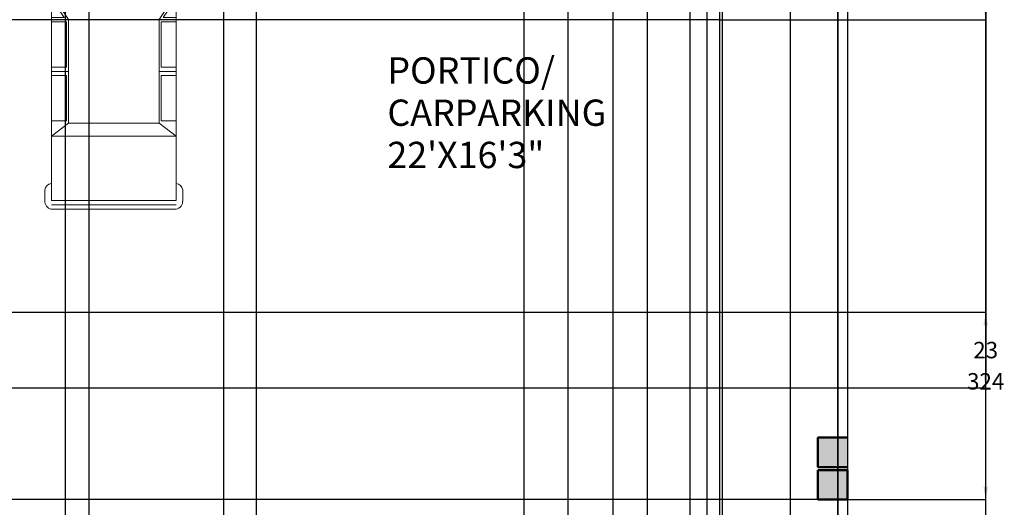
# Model space of a CAD drawing. Units: inches. Extents: x 460 to 1030, y -658 to 271.
# Tile 5 of 10: x 728 to 1028, y -488 to -340. Entities that reach past the tile are written whole.
import ezdxf

# ---------------------------------------------------------------- set-up
doc = ezdxf.new("R2010")
doc.units = ezdxf.units.IN
doc.header["$MEASUREMENT"] = 0
doc.linetypes.add('ACAD_ISO02W100', pattern=[15, 12, -3])
for name, color, linetype, lineweight in [('A-ANNO-DIMS', 2, 'Continuous', 18), ('A-AREA-IDEN', 7, 'Continuous', 25), ('A-COLS', 7, 'Continuous', 50), ('A-ROOF-OVHD', 8, 'ACAD_ISO02W100', 18), ('C-PROP', 7, 'Continuous', 25), ('C-SITE-VEHI', 8, 'Continuous', 13)]:
    doc.layers.add(name, color=color, linetype=linetype, lineweight=lineweight)
doc.layers.add('A-COLS-PATT', color=7, linetype='Continuous', lineweight=13, true_color=0xffffff)
doc.styles.get("Standard").update_dxf_attribs({"font": 'arial.ttf'})
doc.dimstyles.get("Standard").update_dxf_attribs({"dimtxt": 5, "dimasz": 4, "dimexe": 0.18, "dimexo": 0.0625, "dimgap": 0.09, "dimtad": 0, "dimtih": 1, "dimtoh": 1, "dimdec": 1, "dimzin": 0, "dimdsep": 46, "dimlunit": 4, "dimtxsty": 'Standard', "dimcen": 0.09, "dimadec": 0, "dimazin": 0, "dimtfac": 1, "dimtdec": 1, "dimtofl": 0, "dimtmove": 0, "dimatfit": 3, "dimfxl": 1, "dimtolj": 1, "dimtzin": 0, "dimarcsym": 0})

# ---------------------------------------------------------------- blocks, each defined once
blk = doc.blocks.new('*U14')
for p, q in [((3, -10), (3, 974)), ((70, -10), (70, 973)), ((138, 1075), (308, 1075)), ((138, 973), (410, 973)), ((138, -10), (138, 971)), ((410, 973), (4581, 973)), ((1563, -10), (1563, 973)), ((1563, 973), (1969, 702)), ((1630, 973), (1936, 769)), ((1936, 769), (1936, 973)), ((2003, 973), (2003, 736)), ((2716, 736), (2716, 973)), ((2783, 702), (2783, 973)), ((2851, 973), (2851, 736)), ((3563, 736), (3563, 973)), ((3597, 702), (3801, 973)), ((3801, -10), (3801, 973)), ((4818, 973), (4547, 973)), ((4818, 1075), (4649, 1075)), ((4818, -10), (4818, 971)), ((4886, -10), (4886, 973)), ((4954, -10), (4954, 974)), ((1969, 702), (3597, 702)), ((1969, -10), (1969, 702)), ((2003, 736), (2716, 736)), ((2851, 736), (3563, 736)), ((3597, -10), (3597, 702)), ((138, 193), (1563, 396)), ((3, -11), (3, -995)), ((70, -10), (70, -994)), ((138, -11), (138, -992)), ((1563, -10), (1563, -994)), ((1969, -10), (1969, -723)), ((3597, -10), (3597, -723)), ((3801, -10), (3801, -994)), ((4818, -11), (4818, -992)), ((4886, -10), (4886, -994)), ((4954, -11), (4954, -995)), ((138, -214), (1563, -417)), ((1563, -994), (1969, -723)), ((1969, -723), (3597, -723)), ((2003, -994), (2003, -757)), ((2003, -757), (2716, -757)), ((2716, -757), (2716, -994)), ((2783, -723), (2783, -994)), ((2851, -757), (3563, -757)), ((2851, -994), (2851, -757)), ((3563, -757), (3563, -994)), ((3597, -723), (3801, -994)), ((1630, -994), (1936, -790)), ((1936, -790), (1936, -994)), ((138, -994), (410, -994)), ((410, -994), (4581, -994)), ((4818, -994), (4547, -994)), ((138, -1096), (308, -1096)), ((4818, -1096), (4649, -1096))]:
    blk.add_line(p, q)
for centre, radius, start, end in [((128, 946), 129, 85.6455, 168.0943), ((291, 956), 120, 8.1301, 81.87), ((4665, 956), 120, 98.13, 171.8699), ((4828, 946), 129, 11.9057, 94.3545), ((128, -967), 129, 191.9057, 274.3545), ((291, -977), 120, 278.13, 351.8699), ((4665, -977), 120, 188.1301, 261.87), ((4828, -967), 129, 265.6455, 348.0943)]:
    blk.add_arc(centre, radius, start, end)
blk = doc.blocks.new('*D42')
at = {"layer": 'A-ANNO-DIMS', "color": 0, "lineweight": -2, "transparency": 16777216}
for p, q in [((940.86, -287.73), (1022.03, -287.73)), ((1021.85, -291.73), (1021.85, -447.08)), ((1021.85, -607.73), (1021.85, -452.37)), ((979.86, -611.73), (1022.03, -611.73))]:
    blk.add_line(p, q, dxfattribs=at)
at = {"layer": 'A-ANNO-DIMS', "color": 0, "transparency": 16777216}
for points in [[(1021.18, -291.73), (1022.51, -291.73), (1021.85, -287.73)], [(1021.18, -607.73), (1022.51, -607.73), (1021.85, -611.73)]]:
    blk.add_solid(points, dxfattribs=at)
at = {"layer": 'Defpoints', "color": 0, "transparency": 16777216}
for p in [(940.8, -287.73), (1021.85, -287.73), (979.8, -611.73)]:
    blk.add_point(p, dxfattribs=at)
at = {"layer": 'A-ANNO-DIMS', "color": 0, "transparency": 16777216, "insert": (1021.85, -449.73), "char_height": 5, "attachment_point": 5}
blk.add_mtext('\\A1;324', dxfattribs=at)
blk = doc.blocks.new('*D44')
at = {"layer": 'A-ANNO-DIMS', "color": 0, "lineweight": -2, "transparency": 16777216}
for p, q in [((940.86, 90.27), (1022.03, 90.27)), ((1021.85, 86.27), (1021.85, -195.08)), ((1021.85, -481.73), (1021.85, -200.37)), ((979.86, -485.73), (1022.03, -485.73))]:
    blk.add_line(p, q, dxfattribs=at)
at = {"layer": 'A-ANNO-DIMS', "color": 0, "transparency": 16777216}
for points in [[(1021.18, 86.27), (1022.51, 86.27), (1021.85, 90.27)], [(1021.18, -481.73), (1022.51, -481.73), (1021.85, -485.73)]]:
    blk.add_solid(points, dxfattribs=at)
at = {"layer": 'Defpoints', "color": 0, "transparency": 16777216}
for p in [(940.8, 90.27), (979.8, -485.73), (1021.85, -485.73)]:
    blk.add_point(p, dxfattribs=at)
at = {"layer": 'A-ANNO-DIMS', "color": 0, "transparency": 16777216, "insert": (1021.85, -197.73), "char_height": 5, "attachment_point": 5}
blk.add_mtext('\\A1;576', dxfattribs=at)
blk = doc.blocks.new('*D45')
at = {"layer": 'A-ANNO-DIMS', "color": 0, "lineweight": -2, "transparency": 16777216}
for p, q in [((976.8, 126.21), (976.8, -654.61)), ((940.8, 90.21), (940.8, -654.61)), ((944.8, -654.43), (955.13, -654.43)), ((972.8, -654.43), (962.46, -654.43))]:
    blk.add_line(p, q, dxfattribs=at)
at = {"layer": 'A-ANNO-DIMS', "color": 0, "transparency": 16777216}
for points in [[(944.8, -653.77), (944.8, -655.1), (940.8, -654.43)], [(972.8, -653.77), (972.8, -655.1), (976.8, -654.43)]]:
    blk.add_solid(points, dxfattribs=at)
at = {"layer": 'Defpoints', "color": 0, "transparency": 16777216}
for p in [(976.8, 126.27), (940.8, 90.27), (976.8, -654.43)]:
    blk.add_point(p, dxfattribs=at)
at = {"layer": 'A-ANNO-DIMS', "color": 0, "transparency": 16777216, "insert": (958.8, -654.43), "char_height": 5, "attachment_point": 5}
blk.add_mtext('\\A1;36', dxfattribs=at)
blk = doc.blocks.new('*D46')
at = {"layer": 'A-ANNO-DIMS', "color": 0, "lineweight": -2, "transparency": 16777216}
for p, q in [((936.98, 127.21), (936.98, -654.61)), ((962.32, 127.21), (962.32, -654.61)), ((932.98, -654.43), (928.98, -654.43)), ((966.32, -654.43), (970.32, -654.43))]:
    blk.add_line(p, q, dxfattribs=at)
at = {"layer": 'A-ANNO-DIMS', "color": 0, "transparency": 16777216}
for points in [[(932.98, -653.77), (932.98, -655.1), (936.98, -654.43)], [(966.32, -653.77), (966.32, -655.1), (962.32, -654.43)]]:
    blk.add_solid(points, dxfattribs=at)
at = {"layer": 'Defpoints', "color": 0, "transparency": 16777216}
for p in [(936.98, 127.27), (962.32, 127.27), (962.32, -654.43)]:
    blk.add_point(p, dxfattribs=at)
at = {"layer": 'A-ANNO-DIMS', "color": 0, "transparency": 16777216, "insert": (949.65, -654.43), "char_height": 5, "attachment_point": 5}
blk.add_mtext('\\A1;25.346', dxfattribs=at)
blk = doc.blocks.new('*D47')
at = {"layer": 'A-ANNO-DIMS', "color": 0, "lineweight": -2, "transparency": 16777216}
for p, q in [((962.32, 129.21), (962.32, -654.61)), ((979.8, 129.21), (979.8, -654.61)), ((966.32, -654.43), (975.8, -654.43)), ((979.8, -654.43), (983.8, -654.43))]:
    blk.add_line(p, q, dxfattribs=at)
at = {"layer": 'A-ANNO-DIMS', "color": 0, "transparency": 16777216}
for points in [[(966.32, -653.77), (966.32, -655.1), (962.32, -654.43)], [(975.8, -653.77), (975.8, -655.1), (979.8, -654.43)]]:
    blk.add_solid(points, dxfattribs=at)
at = {"layer": 'Defpoints', "color": 0, "transparency": 16777216}
for p in [(962.32, 129.27), (979.8, 129.27), (979.8, -654.43)]:
    blk.add_point(p, dxfattribs=at)
at = {"layer": 'A-ANNO-DIMS', "color": 0, "transparency": 16777216, "insert": (994.02, -654.43), "char_height": 5, "attachment_point": 5}
blk.add_mtext('\\A1;17.474', dxfattribs=at)
blk = doc.blocks.new('*D48')
at = {"layer": 'A-ANNO-DIMS', "color": 0, "lineweight": -2, "transparency": 16777216}
for p, q in [((799.88, -611.66), (799.88, 267.89)), ((803.88, 267.71), (860.58, 267.71)), ((937.7, 267.71), (881, 267.71)), ((941.7, -611.66), (941.7, 267.89))]:
    blk.add_line(p, q, dxfattribs=at)
at = {"layer": 'A-ANNO-DIMS', "color": 0, "transparency": 16777216}
for points in [[(803.88, 268.38), (803.88, 267.04), (799.88, 267.71)], [(937.7, 268.38), (937.7, 267.04), (941.7, 267.71)]]:
    blk.add_solid(points, dxfattribs=at)
at = {"layer": 'Defpoints', "color": 0, "transparency": 16777216}
for p in [(941.7, 267.71), (799.88, -611.73), (941.7, -611.73)]:
    blk.add_point(p, dxfattribs=at)
at = {"layer": 'A-ANNO-DIMS', "color": 0, "transparency": 16777216, "insert": (870.79, 267.71), "char_height": 5, "attachment_point": 5}
blk.add_mtext('\\A1;141.82', dxfattribs=at)
blk = doc.blocks.new('*D49')
at = {"layer": 'A-ANNO-DIMS', "color": 0, "lineweight": -2, "transparency": 16777216}
for p, q in [((941.7, -608.66), (941.7, 267.89)), ((945.7, 267.71), (953.15, 267.71)), ((972.8, 267.71), (965.35, 267.71)), ((976.8, -608.66), (976.8, 267.89))]:
    blk.add_line(p, q, dxfattribs=at)
at = {"layer": 'A-ANNO-DIMS', "color": 0, "transparency": 16777216}
for points in [[(945.7, 268.38), (945.7, 267.04), (941.7, 267.71)], [(972.8, 268.38), (972.8, 267.04), (976.8, 267.71)]]:
    blk.add_solid(points, dxfattribs=at)
at = {"layer": 'Defpoints', "color": 0, "transparency": 16777216}
for p in [(976.8, 267.71), (941.7, -608.73), (976.8, -608.73)]:
    blk.add_point(p, dxfattribs=at)
at = {"layer": 'A-ANNO-DIMS', "color": 0, "transparency": 16777216, "insert": (959.25, 267.71), "char_height": 5, "attachment_point": 5}
blk.add_mtext('\\A1;35.1', dxfattribs=at)
blk = doc.blocks.new('*D50')
at = {"layer": 'A-ANNO-DIMS', "color": 0, "lineweight": -2, "transparency": 16777216}
for p, q in [((700.86, -428.73), (1022.03, -428.73)), ((1021.85, -432.73), (1021.85, -437.58)), ((1021.85, -447.73), (1021.85, -442.87)), ((710.38, -451.73), (1022.03, -451.73))]:
    blk.add_line(p, q, dxfattribs=at)
at = {"layer": 'A-ANNO-DIMS', "color": 0, "transparency": 16777216}
for points in [[(1021.18, -432.73), (1022.51, -432.73), (1021.85, -428.73)], [(1021.18, -447.73), (1022.51, -447.73), (1021.85, -451.73)]]:
    blk.add_solid(points, dxfattribs=at)
at = {"layer": 'Defpoints', "color": 0, "transparency": 16777216}
for p in [(700.8, -428.73), (710.32, -451.73), (1021.85, -451.73)]:
    blk.add_point(p, dxfattribs=at)
at = {"layer": 'A-ANNO-DIMS', "color": 0, "transparency": 16777216, "insert": (1021.85, -440.23), "char_height": 5, "attachment_point": 5}
blk.add_mtext('\\A1;23', dxfattribs=at)
blk = doc.blocks.new('*D53')
at = {"layer": 'A-ANNO-DIMS', "color": 0, "lineweight": -2, "transparency": 16777216}
for p, q in [((908.35, -281.79), (908.35, -654.61)), ((931.8, -281.79), (931.8, -654.61)), ((904.35, -654.43), (900.35, -654.43)), ((935.8, -654.43), (939.8, -654.43))]:
    blk.add_line(p, q, dxfattribs=at)
at = {"layer": 'A-ANNO-DIMS', "color": 0, "transparency": 16777216}
for points in [[(904.35, -653.77), (904.35, -655.1), (908.35, -654.43)], [(935.8, -653.77), (935.8, -655.1), (931.8, -654.43)]]:
    blk.add_solid(points, dxfattribs=at)
at = {"layer": 'Defpoints', "color": 0, "transparency": 16777216}
for p in [(908.35, -281.73), (931.8, -281.73), (931.8, -654.43)]:
    blk.add_point(p, dxfattribs=at)
at = {"layer": 'A-ANNO-DIMS', "color": 0, "transparency": 16777216, "insert": (920.07, -654.43), "char_height": 5, "attachment_point": 5}
blk.add_mtext('\\A1;23.45', dxfattribs=at)
blk = doc.blocks.new('*D54')
at = {"layer": 'A-ANNO-DIMS', "color": 0, "lineweight": -2, "transparency": 16777216}
for p, q in [((894.61, -141.78), (894.61, -654.61)), ((931.8, -141.78), (931.8, -654.61)), ((898.61, -654.43), (904.68, -654.43)), ((927.8, -654.43), (921.73, -654.43))]:
    blk.add_line(p, q, dxfattribs=at)
at = {"layer": 'A-ANNO-DIMS', "color": 0, "transparency": 16777216}
for points in [[(898.61, -653.77), (898.61, -655.1), (894.61, -654.43)], [(927.8, -653.77), (927.8, -655.1), (931.8, -654.43)]]:
    blk.add_solid(points, dxfattribs=at)
at = {"layer": 'Defpoints', "color": 0, "transparency": 16777216}
for p in [(894.61, -141.72), (931.8, -141.72), (931.8, -654.43)]:
    blk.add_point(p, dxfattribs=at)
at = {"layer": 'A-ANNO-DIMS', "color": 0, "transparency": 16777216, "insert": (913.2, -654.43), "char_height": 5, "attachment_point": 5}
blk.add_mtext('\\A1;37.18', dxfattribs=at)
blk = doc.blocks.new('*D57')
at = {"layer": 'A-ANNO-DIMS', "color": 0, "lineweight": -2, "transparency": 16777216}
for p, q in [((717.53, -38.79), (717.53, -654.61)), ((741.59, -38.79), (741.59, -654.61)), ((713.53, -654.43), (709.53, -654.43)), ((745.59, -654.43), (749.59, -654.43))]:
    blk.add_line(p, q, dxfattribs=at)
at = {"layer": 'A-ANNO-DIMS', "color": 0, "transparency": 16777216}
for points in [[(713.53, -653.77), (713.53, -655.1), (717.53, -654.43)], [(745.59, -653.77), (745.59, -655.1), (741.59, -654.43)]]:
    blk.add_solid(points, dxfattribs=at)
at = {"layer": 'Defpoints', "color": 0, "transparency": 16777216}
for p in [(717.53, -38.73), (741.59, -38.73), (741.59, -654.43)]:
    blk.add_point(p, dxfattribs=at)
at = {"layer": 'A-ANNO-DIMS', "color": 0, "transparency": 16777216, "insert": (729.56, -654.43), "char_height": 5, "attachment_point": 5}
blk.add_mtext('\\A1;24.065', dxfattribs=at)
blk = doc.blocks.new('*D66')
at = {"layer": 'A-ANNO-DIMS', "color": 0, "lineweight": -2, "transparency": 16777216}
for p, q in [((940.73, -339.73), (470.68, -339.73)), ((470.86, -343.73), (470.86, -410.08)), ((470.86, -481.73), (470.86, -415.37)), ((979.73, -485.73), (470.68, -485.73))]:
    blk.add_line(p, q, dxfattribs=at)
at = {"layer": 'A-ANNO-DIMS', "color": 0, "transparency": 16777216}
for points in [[(470.19, -343.73), (471.52, -343.73), (470.86, -339.73)], [(470.19, -481.73), (471.52, -481.73), (470.86, -485.73)]]:
    blk.add_solid(points, dxfattribs=at)
at = {"layer": 'Defpoints', "color": 0, "transparency": 16777216}
for p in [(940.8, -339.73), (470.86, -485.73), (979.8, -485.73)]:
    blk.add_point(p, dxfattribs=at)
at = {"layer": 'A-ANNO-DIMS', "color": 0, "transparency": 16777216, "insert": (470.86, -412.73), "char_height": 5, "attachment_point": 5}
blk.add_mtext('\\A1;146', dxfattribs=at)
blk = doc.blocks.new('*D67')
at = {"layer": 'A-ANNO-DIMS', "color": 0, "lineweight": -2, "transparency": 16777216}
for p, q in [((940.86, -287.73), (1022.03, -287.73)), ((1021.85, -291.73), (1021.85, -311.08)), ((1021.85, -335.73), (1021.85, -316.37)), ((940.86, -339.73), (1022.03, -339.73))]:
    blk.add_line(p, q, dxfattribs=at)
at = {"layer": 'A-ANNO-DIMS', "color": 0, "transparency": 16777216}
for points in [[(1021.18, -291.73), (1022.51, -291.73), (1021.85, -287.73)], [(1021.18, -335.73), (1022.51, -335.73), (1021.85, -339.73)]]:
    blk.add_solid(points, dxfattribs=at)
at = {"layer": 'Defpoints', "color": 0, "transparency": 16777216}
for p in [(940.8, -287.73), (1021.85, -287.73), (940.8, -339.73)]:
    blk.add_point(p, dxfattribs=at)
at = {"layer": 'A-ANNO-DIMS', "color": 0, "transparency": 16777216, "insert": (1021.85, -313.73), "char_height": 5, "attachment_point": 5}
blk.add_mtext('\\A1;52', dxfattribs=at)
blk = doc.blocks.new('*D69')
at = {"layer": 'A-ANNO-DIMS', "color": 0, "lineweight": -2, "transparency": 16777216}
for p, q in [((881.27, 90.21), (881.27, -654.61)), ((918.77, 90.21), (918.77, -654.61)), ((885.27, -654.43), (893.42, -654.43)), ((914.77, -654.43), (906.62, -654.43))]:
    blk.add_line(p, q, dxfattribs=at)
at = {"layer": 'A-ANNO-DIMS', "color": 0, "transparency": 16777216}
for points in [[(885.27, -653.77), (885.27, -655.1), (881.27, -654.43)], [(914.77, -653.77), (914.77, -655.1), (918.77, -654.43)]]:
    blk.add_solid(points, dxfattribs=at)
at = {"layer": 'Defpoints', "color": 0, "transparency": 16777216}
for p in [(881.27, 90.27), (918.77, 90.27), (918.77, -654.43)]:
    blk.add_point(p, dxfattribs=at)
at = {"layer": 'A-ANNO-DIMS', "color": 0, "transparency": 16777216, "insert": (900.02, -654.43), "char_height": 5, "attachment_point": 5}
blk.add_mtext('\\A1;37.5', dxfattribs=at)
blk = doc.blocks.new('*D70')
at = {"layer": 'A-ANNO-DIMS', "color": 0, "lineweight": -2, "transparency": 16777216}
for p, q in [((716.71, -287.79), (716.71, -654.61)), ((789.82, -287.79), (789.82, -654.61)), ((720.71, -654.43), (744.79, -654.43)), ((785.82, -654.43), (761.75, -654.43))]:
    blk.add_line(p, q, dxfattribs=at)
at = {"layer": 'A-ANNO-DIMS', "color": 0, "transparency": 16777216}
for points in [[(720.71, -653.77), (720.71, -655.1), (716.71, -654.43)], [(785.82, -653.77), (785.82, -655.1), (789.82, -654.43)]]:
    blk.add_solid(points, dxfattribs=at)
at = {"layer": 'Defpoints', "color": 0, "transparency": 16777216}
for p in [(716.71, -287.73), (789.82, -287.73), (789.82, -654.43)]:
    blk.add_point(p, dxfattribs=at)
at = {"layer": 'A-ANNO-DIMS', "color": 0, "transparency": 16777216, "insert": (753.27, -654.43), "char_height": 5, "attachment_point": 5}
blk.add_mtext('\\A1;73.12', dxfattribs=at)
blk = doc.blocks.new('*D72')
at = {"layer": 'A-ANNO-DIMS', "color": 0, "lineweight": -2, "transparency": 16777216}
for p, q in [((715.8, 68.25), (715.8, -654.61)), ((748.8, 57.75), (748.8, -654.61)), ((719.8, -654.43), (728.63, -654.43)), ((744.8, -654.43), (735.97, -654.43))]:
    blk.add_line(p, q, dxfattribs=at)
at = {"layer": 'A-ANNO-DIMS', "color": 0, "transparency": 16777216}
for points in [[(719.8, -653.77), (719.8, -655.1), (715.8, -654.43)], [(744.8, -653.77), (744.8, -655.1), (748.8, -654.43)]]:
    blk.add_solid(points, dxfattribs=at)
at = {"layer": 'Defpoints', "color": 0, "transparency": 16777216}
for p in [(715.8, 68.31), (748.8, 57.81), (748.8, -654.43)]:
    blk.add_point(p, dxfattribs=at)
at = {"layer": 'A-ANNO-DIMS', "color": 0, "transparency": 16777216, "insert": (732.3, -654.43), "char_height": 5, "attachment_point": 5}
blk.add_mtext('\\A1;33', dxfattribs=at)

msp = doc.modelspace()

# ---------------------------------------------------------------- hatches: boundary and pattern name
at = {"layer": 'A-COLS-PATT'}
h = msp.add_hatch(color=256, dxfattribs=at)
h.dxf.hatch_style = 1
h.paths.add_polyline_path([(979.7961, -466.833), (970.7961, -466.833), (970.7961, -475.833), (979.7961, -475.833)])
h.paths.add_polyline_path([(979.7961, -476.7262), (970.7961, -476.7262), (970.7961, -485.7262), (979.7961, -485.7262)])

# ---------------------------------------------------------------- linework, layer by layer
at = {"layer": 'A-COLS'}
for p, q in [((970.7961, -466.833), (970.7961, -475.833)), ((979.7961, -466.833), (970.7961, -466.833)), ((979.7961, -475.833), (970.7961, -475.833)), ((979.7961, -476.7262), (970.7961, -476.7262)), ((970.7961, -476.7262), (970.7961, -485.7262)), ((979.7961, -476.7262), (979.7961, -485.7262)), ((979.7961, -485.7262), (970.7961, -485.7262))]:
    msp.add_line(p, q, dxfattribs=at)
at = {"layer": 'A-ROOF-OVHD'}
msp.add_line((976.7961, -485.7262), (700.7961, -485.7262), dxfattribs=at)
at = {"layer": 'C-PROP'}
for p, q in [((979.7961, 129.2738), (979.7961, -524.7262)), ((976.7961, 126.2738), (976.7961, -466.833)), ((976.7961, -485.7262), (976.7961, -608.7262))]:
    msp.add_line(p, q, dxfattribs=at)

# ---------------------------------------------------------------- block references
at = {"layer": 'C-SITE-VEHI', "xscale": 0.0193263137064046, "yscale": 0.0193263137064046, "zscale": 0.0193263137064046, "rotation": 270}
msp.add_blockref('*U14', (756.6242, -301.6472), dxfattribs=at)

# ---------------------------------------------------------------- texts
at = {"layer": 'A-AREA-IDEN'}
for s, p in [('PORTICO/', (839.707, -359.1666)), ('CARPARKING', (839.707, -372.0179)), ('22\'X16\'3"', (839.707, -384.8692))]:
    msp.add_text(s, height=8, dxfattribs=at).set_placement(p)

# ---------------------------------------------------------------- dimensions: what is measured, and where the dimension line sits
at = {"layer": 'A-ANNO-DIMS'}
for base, p1, p2, override, picture, middle in [((941.6978, 267.7108), (799.8801, -611.7262), (941.6978, -611.7262), {"dimdec": 2, "dimlfac": 1, "dimrnd": 0, "dimzin": 0, "dimdsep": 46, "dimlunit": 2}, '*D48', (870.7889, 267.7108)), ((976.7961, 267.7108), (941.6978, -608.7262), (976.7961, -608.7262), {"dimdec": 1, "dimlfac": 1, "dimrnd": 0, "dimzin": 0, "dimdsep": 46, "dimlunit": 2}, '*D49', (959.247, 267.7108)), ((979.7961, -654.4339), (962.3217, 129.2738), (979.7961, 129.2738), {"dimdec": 3, "dimlfac": 1, "dimrnd": 0, "dimzin": 0, "dimdsep": 46, "dimlunit": 2}, '*D47', (994.0191, -654.4339)), ((962.3217, -654.4339), (936.9757, 127.2738), (962.3217, 127.2738), {"dimdec": 3, "dimlfac": 1, "dimrnd": 0, "dimzin": 0, "dimdsep": 46, "dimlunit": 2}, '*D46', (949.6487, -654.4339)), ((976.7961, -654.4339), (940.7961, 90.2738), (976.7961, 126.2738), {"dimdec": 0, "dimlfac": 1, "dimrnd": 0, "dimzin": 0, "dimdsep": 46, "dimlunit": 2}, '*D45', (958.7961, -654.4339)), ((918.7723, -654.4339), (881.2728, 90.2738), (918.7723, 90.2738), {"dimdec": 1, "dimlfac": 1, "dimrnd": 0, "dimzin": 0, "dimdsep": 46, "dimlunit": 2}, '*D69', (900.0226, -654.4339)), ((748.7961, -654.4339), (715.7961, 68.3148), (748.7961, 57.8148), {"dimdec": 0, "dimlfac": 1, "dimrnd": 0, "dimzin": 0, "dimdsep": 46, "dimlunit": 2}, '*D72', (732.2961, -654.4339)), ((741.5908, -654.4339), (717.5258, -38.7262), (741.5908, -38.7262), {"dimdec": 3, "dimlfac": 1, "dimrnd": 0, "dimzin": 0, "dimdsep": 46, "dimlunit": 2}, '*D57', (729.5583, -654.4339)), ((931.7961, -654.4339), (894.6132, -141.7212), (931.7961, -141.7212), {"dimdec": 2, "dimlfac": 1, "dimrnd": 0, "dimzin": 0, "dimdsep": 46, "dimlunit": 2}, '*D54', (913.2047, -654.4339)), ((931.7961, -654.4339), (908.3452, -281.7262), (931.7961, -281.7262), {"dimdec": 2, "dimlfac": 1, "dimrnd": 0, "dimzin": 0, "dimdsep": 46, "dimlunit": 2}, '*D53', (920.0707, -654.4339)), ((789.8237, -654.4339), (716.7073, -287.7262), (789.8237, -287.7262), {"dimdec": 2, "dimlfac": 1, "dimrnd": 0, "dimzin": 0, "dimdsep": 46, "dimlunit": 2}, '*D70', (753.2655, -654.4339))]:
    dim = msp.add_linear_dim(base=base, p1=p1, p2=p2, dimstyle='Standard', override=override, dxfattribs=at)
    dim.commit()
    dim.dimension.update_dxf_attribs({"geometry": picture, "text_midpoint": middle})
for base, p1, p2, picture, middle in [((1021.8461, -485.7262), (940.7961, 90.2738), (979.7961, -485.7262), '*D44', (1021.8461, -197.7262)), ((1021.8461, -287.7262), (979.7961, -611.7262), (940.7961, -287.7262), '*D42', (1021.8461, -449.7262)), ((1021.8461, -287.7262), (940.7961, -339.7262), (940.7961, -287.7262), '*D67', (1021.8461, -313.7262)), ((470.8563, -485.7262), (940.7961, -339.7262), (979.7961, -485.7262), '*D66', (470.8563, -412.7262)), ((1021.8461, -451.7262), (700.7961, -428.7262), (710.3211, -451.7262), '*D50', (1021.8461, -440.2262))]:
    dim = msp.add_linear_dim(base=base, p1=p1, p2=p2, angle=90, dimstyle='Standard', override={"dimdec": 0, "dimlfac": 1, "dimrnd": 0, "dimzin": 0, "dimdsep": 46, "dimlunit": 2}, dxfattribs=at)
    dim.commit()
    dim.dimension.update_dxf_attribs({"geometry": picture, "text_midpoint": middle})

doc.saveas('drawing.dxf')
